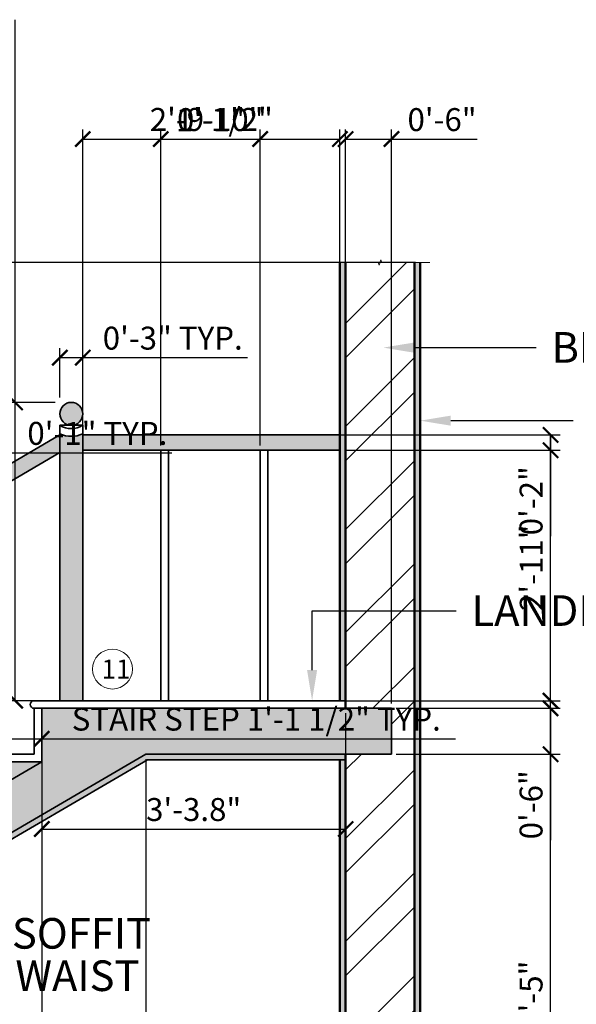
# Model space of a CAD drawing. Units: inches. Extents: x 2205 to 2524, y 4609 to 4803.
# Tile 4 of 5: x 2377 to 2450, y 4674 to 4803. Entities that reach past the tile are written whole.
import ezdxf
from ezdxf import colors
from ezdxf.entities.mleader import LeaderData, LeaderLine
from ezdxf.math import Vec2, Vec3

# ---------------------------------------------------------------- set-up
doc = ezdxf.new("R2010")
doc.units = ezdxf.units.IN
for name, color, linetype, lineweight in [('A-ANNO-DIMS', 2, 'Continuous', 18), ('A-ANNO-SYMB', 3, 'Continuous', 18), ('A-ANNO-TEXT', 7, 'Continuous', 18), ('A-FLOR-STRS', 7, 'Continuous', 35), ('A-SECT-PATT', 252, 'Continuous', 13), ('A-WALL', 1, 'Continuous', 50), ('A-WALL-PATT', 8, 'Continuous', 13), ('S-BEAM', 3, 'Continuous', 35)]:
    doc.layers.add(name, color=color, linetype=linetype, lineweight=lineweight)
doc.styles.get("Standard").update_dxf_attribs({"font": 'arial.ttf'})
doc.dimstyles.new('ISO-25', dxfattribs={"dimtxt": 3, "dimasz": 2, "dimexe": 1.25, "dimexo": 0.625, "dimtad": 1, "dimdec": 1, "dimlunit": 3, "dimtxsty": 'Standard', "dimblk": 'ARCHTICK', "dimcen": 2.5, "dimclrd": 5, "dimclre": 2, "dimclrt": 6, "dimadec": 0, "dimazin": 0, "dimtfac": 1, "dimtdec": 1, "dimtmove": 0, "dimatfit": 3, "dimfxl": 1, "dimarcsym": 0})

# ---------------------------------------------------------------- blocks, each defined once
blk = doc.blocks.new('_ArchTick')
at = {"color": 0, "linetype": 'ByBlock', "const_width": 0.15}
blk.add_lwpolyline([(-0.5, -0.5), (0.5, 0.5)], dxfattribs=at)
blk = doc.blocks.new('*D4')
at = {"layer": 'A-ANNO-DIMS', "color": 0, "lineweight": -2, "transparency": 16777216}
for p, q in [((2379.7, 4712.35), (2379.7, 4695.95)), ((2419.45, 4712.35), (2419.45, 4695.95)), ((2379.7, 4697.2), (2419.45, 4697.2))]:
    blk.add_line(p, q, dxfattribs=at)
at = {"layer": 'DEFPOINTS', "color": 0, "transparency": 16777216}
for p in [(2379.7, 4712.98), (2419.45, 4712.98), (2419.45, 4697.2)]:
    blk.add_point(p, dxfattribs=at)
at = {"layer": 'A-ANNO-DIMS', "color": 0, "lineweight": -2, "transparency": 16777216, "xscale": 2, "yscale": 2, "zscale": 2, "rotation": 180}
blk.add_blockref('_ArchTick', (2379.7, 4697.2), dxfattribs=at)
at = {"layer": 'A-ANNO-DIMS', "color": 0, "lineweight": -2, "transparency": 16777216, "xscale": 2, "yscale": 2, "zscale": 2}
blk.add_blockref('_ArchTick', (2419.45, 4697.2), dxfattribs=at)
at = {"layer": 'A-ANNO-DIMS', "color": 0, "transparency": 16777216, "insert": (2399.57, 4699.36), "char_height": 3, "attachment_point": 5}
blk.add_mtext('3\'-3.8"', dxfattribs=at)
blk = doc.blocks.new('STAIR-STEP')
for p, q in [((2282.7, 4650.98), (2270.7, 4650.98)), ((2283.7, 4649.98), (2270.7, 4649.98)), ((2270.7, 4649.98), (2270.7, 4642.98)), ((2271.7, 4649.98), (2271.7, 4642.98))]:
    blk.add_line(p, q)
blk.add_arc((2270.7, 4650.48), 0.5, 90, 270)
blk = doc.blocks.new('NEWEL-POST')
for p, q in [((2261.7, 4679.98), (2261.7, 4643.98)), ((2261.71, 4679.98), (2261.7, 4679.98)), ((2261.71, 4679.98), (2264.69, 4679.98)), ((2264.7, 4679.98), (2264.69, 4679.98)), ((2264.7, 4679.98), (2264.7, 4643.98))]:
    blk.add_line(p, q)
blk.add_circle((2263.2, 4681.48), 1.5)
for radius, start, end in [(2.78, 237.6128, 302.3872), (3.78, 246.6124, 293.3876)]:
    blk.add_arc((2263.2, 4682.33), radius, start, end)
blk = doc.blocks.new('*D9')
at = {"layer": 'A-ANNO-DIMS', "color": 2, "lineweight": -2, "transparency": 16777216}
for p, q in [((2366.2, 4707.6), (2366.2, 4710.25)), ((2379.7, 4707.6), (2379.7, 4710.25))]:
    blk.add_line(p, q, dxfattribs=at)
at = {"layer": 'A-ANNO-DIMS', "color": 5, "lineweight": -2, "transparency": 16777216}
for p, q in [((2366.2, 4709), (2379.7, 4709)), ((2379.7, 4709), (2433.83, 4709))]:
    blk.add_line(p, q, dxfattribs=at)
at = {"layer": 'DEFPOINTS', "color": 0, "transparency": 16777216}
for p in [(2379.7, 4709), (2366.2, 4706.98), (2379.7, 4706.98)]:
    blk.add_point(p, dxfattribs=at)
at = {"layer": 'A-ANNO-DIMS', "color": 5, "lineweight": -2, "transparency": 16777216, "xscale": 2, "yscale": 2, "zscale": 2, "rotation": 180}
blk.add_blockref('_ArchTick', (2366.2, 4709), dxfattribs=at)
at = {"layer": 'A-ANNO-DIMS', "color": 5, "lineweight": -2, "transparency": 16777216, "xscale": 2, "yscale": 2, "zscale": 2}
blk.add_blockref('_ArchTick', (2379.7, 4709), dxfattribs=at)
at = {"layer": 'A-ANNO-DIMS', "color": 6, "transparency": 16777216, "insert": (2407.76, 4711.18), "char_height": 3, "attachment_point": 5}
blk.add_mtext('STAIR STEP 1\'-1 1/2" TYP.', dxfattribs=at)
blk = doc.blocks.new('*D12')
at = {"layer": 'A-ANNO-DIMS', "color": 2, "lineweight": -2, "transparency": 16777216}
for p, q in [((2372.2, 4741.87), (2372.2, 4747.64)), ((2373.2, 4741.87), (2373.2, 4747.64))]:
    blk.add_line(p, q, dxfattribs=at)
at = {"layer": 'A-ANNO-DIMS', "color": 5, "lineweight": -2, "transparency": 16777216}
for p, q in [((2372.2, 4746.39), (2370.2, 4746.39)), ((2372.2, 4746.39), (2373.2, 4746.39)), ((2373.2, 4746.39), (2396.73, 4746.39))]:
    blk.add_line(p, q, dxfattribs=at)
at = {"layer": 'DEFPOINTS', "color": 0, "transparency": 16777216}
for p in [(2373.2, 4746.39), (2372.2, 4741.25), (2373.2, 4741.25)]:
    blk.add_point(p, dxfattribs=at)
at = {"layer": 'A-ANNO-DIMS', "color": 5, "lineweight": -2, "transparency": 16777216, "xscale": 2, "yscale": 2, "zscale": 2}
blk.add_blockref('_ArchTick', (2372.2, 4746.39), dxfattribs=at)
at = {"layer": 'A-ANNO-DIMS', "color": 5, "lineweight": -2, "transparency": 16777216, "xscale": 2, "yscale": 2, "zscale": 2, "rotation": 180}
blk.add_blockref('_ArchTick', (2373.2, 4746.39), dxfattribs=at)
at = {"layer": 'A-ANNO-DIMS', "color": 6, "transparency": 16777216, "insert": (2386.97, 4748.54), "char_height": 3, "attachment_point": 5}
blk.add_mtext('0\'-1" TYP.', dxfattribs=at)
blk = doc.blocks.new('*D13')
at = {"layer": 'A-ANNO-DIMS', "color": 5, "lineweight": -2, "transparency": 16777216}
for p, q in [((2376.21, 4752.98), (2376.21, 4803.01)), ((2376.21, 4713.98), (2376.21, 4752.98))]:
    blk.add_line(p, q, dxfattribs=at)
at = {"layer": 'A-ANNO-DIMS', "color": 2, "lineweight": -2, "transparency": 16777216}
for p, q in [((2381.44, 4752.98), (2374.96, 4752.98)), ((2381.44, 4713.98), (2374.96, 4713.98))]:
    blk.add_line(p, q, dxfattribs=at)
at = {"layer": 'DEFPOINTS', "color": 0, "transparency": 16777216}
for p in [(2376.21, 4752.98), (2382.06, 4752.98), (2382.06, 4713.98)]:
    blk.add_point(p, dxfattribs=at)
at = {"layer": 'A-ANNO-DIMS', "color": 5, "lineweight": -2, "transparency": 16777216, "xscale": 2, "yscale": 2, "zscale": 2}
for p, rotation in [((2376.21, 4752.98), 90), ((2376.21, 4713.98), 270)]:
    blk.add_blockref('_ArchTick', p, dxfattribs=dict(at, rotation=rotation))
at = {"layer": 'A-ANNO-DIMS', "color": 6, "transparency": 16777216, "insert": (2374.03, 4779), "char_height": 3, "attachment_point": 5, "rotation": 90}
blk.add_mtext('NEWEL POST 3\'-3" TYP.', dxfattribs=at)
blk = doc.blocks.new('*D14')
at = {"layer": 'A-ANNO-DIMS', "color": 2, "lineweight": -2, "transparency": 16777216}
for p, q in [((2382.06, 4753.6), (2382.06, 4760.08)), ((2385.06, 4753.6), (2385.06, 4760.08))]:
    blk.add_line(p, q, dxfattribs=at)
at = {"layer": 'A-ANNO-DIMS', "color": 5, "lineweight": -2, "transparency": 16777216}
for p, q in [((2382.06, 4758.83), (2385.06, 4758.83)), ((2385.06, 4758.83), (2406.6, 4758.83))]:
    blk.add_line(p, q, dxfattribs=at)
at = {"layer": 'DEFPOINTS', "color": 0, "transparency": 16777216}
for p in [(2385.06, 4758.83), (2382.06, 4752.98), (2385.06, 4752.98)]:
    blk.add_point(p, dxfattribs=at)
at = {"layer": 'A-ANNO-DIMS', "color": 5, "lineweight": -2, "transparency": 16777216, "xscale": 2, "yscale": 2, "zscale": 2, "rotation": 180}
blk.add_blockref('_ArchTick', (2382.06, 4758.83), dxfattribs=at)
at = {"layer": 'A-ANNO-DIMS', "color": 5, "lineweight": -2, "transparency": 16777216, "xscale": 2, "yscale": 2, "zscale": 2}
blk.add_blockref('_ArchTick', (2385.06, 4758.83), dxfattribs=at)
at = {"layer": 'A-ANNO-DIMS', "color": 6, "transparency": 16777216, "insert": (2396.83, 4760.99), "char_height": 3, "attachment_point": 5}
blk.add_mtext('0\'-3" TYP.', dxfattribs=at)
blk = doc.blocks.new('*D16')
at = {"layer": 'A-ANNO-DIMS', "color": 2, "lineweight": -2, "transparency": 16777216}
for p, q in [((2428.57, 4771.26), (2222.09, 4771.26)), ((2428.57, 4636.98), (2222.09, 4636.98))]:
    blk.add_line(p, q, dxfattribs=at)
at = {"layer": 'A-ANNO-DIMS', "color": 5, "lineweight": -2, "transparency": 16777216}
blk.add_line((2223.34, 4636.98), (2223.34, 4771.26), dxfattribs=at)
at = {"layer": 'DEFPOINTS', "color": 0, "transparency": 16777216}
for p in [(2223.34, 4771.26), (2429.2, 4771.26), (2429.2, 4636.98)]:
    blk.add_point(p, dxfattribs=at)
at = {"layer": 'A-ANNO-DIMS', "color": 5, "lineweight": -2, "transparency": 16777216, "xscale": 2, "yscale": 2, "zscale": 2}
for p, rotation in [((2223.34, 4771.26), 90), ((2223.34, 4636.98), 270)]:
    blk.add_blockref('_ArchTick', p, dxfattribs=dict(at, rotation=rotation))
at = {"layer": 'A-ANNO-DIMS', "color": 6, "transparency": 16777216, "insert": (2221.17, 4704.12), "char_height": 3, "attachment_point": 5, "rotation": 90}
blk.add_mtext('11\'-2 1/2"', dxfattribs=at)
blk = doc.blocks.new('*D17')
at = {"layer": 'A-ANNO-DIMS', "color": 2, "lineweight": -2, "transparency": 16777216}
for p, q in [((2420.07, 4713.98), (2447.5, 4713.98)), ((2420.07, 4636.98), (2447.5, 4636.98))]:
    blk.add_line(p, q, dxfattribs=at)
at = {"layer": 'A-ANNO-DIMS', "color": 5, "lineweight": -2, "transparency": 16777216}
blk.add_line((2446.25, 4636.98), (2446.25, 4713.98), dxfattribs=at)
at = {"layer": 'DEFPOINTS', "color": 0, "transparency": 16777216}
for p in [(2419.45, 4713.98), (2446.25, 4713.98), (2419.45, 4636.98)]:
    blk.add_point(p, dxfattribs=at)
at = {"layer": 'A-ANNO-DIMS', "color": 5, "lineweight": -2, "transparency": 16777216, "xscale": 2, "yscale": 2, "zscale": 2}
for p, rotation in [((2446.25, 4713.98), 90), ((2446.25, 4636.98), 270)]:
    blk.add_blockref('_ArchTick', p, dxfattribs=dict(at, rotation=rotation))
at = {"layer": 'A-ANNO-DIMS', "color": 6, "transparency": 16777216, "insert": (2444.09, 4675.48), "char_height": 3, "attachment_point": 5, "rotation": 90}
blk.add_mtext('6\'-5"', dxfattribs=at)
blk = doc.blocks.new('*D19')
at = {"layer": 'A-ANNO-DIMS', "color": 2, "lineweight": -2, "transparency": 16777216}
for p, q in [((2426.07, 4712.98), (2447.5, 4712.98)), ((2426.07, 4706.98), (2447.5, 4706.98))]:
    blk.add_line(p, q, dxfattribs=at)
at = {"layer": 'A-ANNO-DIMS', "color": 5, "lineweight": -2, "transparency": 16777216}
for p, q in [((2446.25, 4712.98), (2446.25, 4706.98)), ((2446.25, 4706.98), (2446.25, 4695.75))]:
    blk.add_line(p, q, dxfattribs=at)
at = {"layer": 'DEFPOINTS', "color": 0, "transparency": 16777216}
for p in [(2425.45, 4712.98), (2425.45, 4706.98), (2446.25, 4706.98)]:
    blk.add_point(p, dxfattribs=at)
at = {"layer": 'A-ANNO-DIMS', "color": 5, "lineweight": -2, "transparency": 16777216, "xscale": 2, "yscale": 2, "zscale": 2}
for p, rotation in [((2446.25, 4712.98), 90), ((2446.25, 4706.98), 270)]:
    blk.add_blockref('_ArchTick', p, dxfattribs=dict(at, rotation=rotation))
at = {"layer": 'A-ANNO-DIMS', "color": 6, "transparency": 16777216, "insert": (2444.09, 4700.37), "char_height": 3, "attachment_point": 5, "rotation": 90}
blk.add_mtext('0\'-6"', dxfattribs=at)
blk = doc.blocks.new('*D20')
at = {"layer": 'A-ANNO-DIMS', "color": 2, "lineweight": -2, "transparency": 16777216}
for p, q in [((2419.45, 4713.6), (2419.45, 4788.66)), ((2425.45, 4713.6), (2425.45, 4788.66))]:
    blk.add_line(p, q, dxfattribs=at)
at = {"layer": 'A-ANNO-DIMS', "color": 5, "lineweight": -2, "transparency": 16777216}
for p, q in [((2419.45, 4787.41), (2425.45, 4787.41)), ((2425.45, 4787.41), (2436.67, 4787.41))]:
    blk.add_line(p, q, dxfattribs=at)
at = {"layer": 'DEFPOINTS', "color": 0, "transparency": 16777216}
for p in [(2425.45, 4787.41), (2419.45, 4712.98), (2425.45, 4712.98)]:
    blk.add_point(p, dxfattribs=at)
at = {"layer": 'A-ANNO-DIMS', "color": 5, "lineweight": -2, "transparency": 16777216, "xscale": 2, "yscale": 2, "zscale": 2, "rotation": 180}
blk.add_blockref('_ArchTick', (2419.45, 4787.41), dxfattribs=at)
at = {"layer": 'A-ANNO-DIMS', "color": 5, "lineweight": -2, "transparency": 16777216, "xscale": 2, "yscale": 2, "zscale": 2}
blk.add_blockref('_ArchTick', (2425.45, 4787.41), dxfattribs=at)
at = {"layer": 'A-ANNO-DIMS', "color": 6, "transparency": 16777216, "insert": (2432.06, 4789.56), "char_height": 3, "attachment_point": 5}
blk.add_mtext('0\'-6"', dxfattribs=at)
blk = doc.blocks.new('*D21')
at = {"layer": 'A-ANNO-DIMS', "color": 2, "lineweight": -2, "transparency": 16777216}
for p, q in [((2379.7, 4705.35), (2379.7, 4619.93)), ((2393.32, 4706.35), (2393.32, 4619.93))]:
    blk.add_line(p, q, dxfattribs=at)
at = {"layer": 'A-ANNO-DIMS', "color": 5, "lineweight": -2, "transparency": 16777216}
for p, q in [((2379.7, 4621.18), (2393.32, 4621.18)), ((2393.32, 4621.18), (2411.25, 4621.18))]:
    blk.add_line(p, q, dxfattribs=at)
at = {"layer": 'DEFPOINTS', "color": 0, "transparency": 16777216}
for p in [(2393.32, 4706.98), (2379.7, 4705.98), (2393.32, 4621.18)]:
    blk.add_point(p, dxfattribs=at)
at = {"layer": 'A-ANNO-DIMS', "color": 5, "lineweight": -2, "transparency": 16777216, "xscale": 2, "yscale": 2, "zscale": 2, "rotation": 180}
blk.add_blockref('_ArchTick', (2379.7, 4621.18), dxfattribs=at)
at = {"layer": 'A-ANNO-DIMS', "color": 5, "lineweight": -2, "transparency": 16777216, "xscale": 2, "yscale": 2, "zscale": 2}
blk.add_blockref('_ArchTick', (2393.32, 4621.18), dxfattribs=at)
at = {"layer": 'A-ANNO-DIMS', "color": 6, "transparency": 16777216, "insert": (2403.29, 4623.36), "char_height": 3, "attachment_point": 5}
blk.add_mtext('1\'-1 1/2"', dxfattribs=at)
blk = doc.blocks.new('*D22')
at = {"layer": 'A-ANNO-DIMS', "color": 2, "lineweight": -2, "transparency": 16777216}
for p, q in [((2385.69, 4748.73), (2447.5, 4748.73)), ((2385.69, 4713.98), (2447.5, 4713.98))]:
    blk.add_line(p, q, dxfattribs=at)
at = {"layer": 'A-ANNO-DIMS', "color": 5, "lineweight": -2, "transparency": 16777216}
blk.add_line((2446.25, 4713.98), (2446.25, 4748.73), dxfattribs=at)
at = {"layer": 'DEFPOINTS', "color": 0, "transparency": 16777216}
for p in [(2385.06, 4748.73), (2446.25, 4748.73), (2385.06, 4713.98)]:
    blk.add_point(p, dxfattribs=at)
at = {"layer": 'A-ANNO-DIMS', "color": 5, "lineweight": -2, "transparency": 16777216, "xscale": 2, "yscale": 2, "zscale": 2}
for p, rotation in [((2446.25, 4748.73), 90), ((2446.25, 4713.98), 270)]:
    blk.add_blockref('_ArchTick', p, dxfattribs=dict(at, rotation=rotation))
at = {"layer": 'A-ANNO-DIMS', "color": 6, "transparency": 16777216, "insert": (2444.12, 4731.36), "char_height": 3, "attachment_point": 5, "rotation": 90}
blk.add_mtext('2\'-11"', dxfattribs=at)
blk = doc.blocks.new('*D23')
at = {"layer": 'A-ANNO-DIMS', "color": 2, "lineweight": -2, "transparency": 16777216}
for p, q in [((2419.32, 4748.73), (2447.5, 4748.73)), ((2419.32, 4746.73), (2447.5, 4746.73))]:
    blk.add_line(p, q, dxfattribs=at)
at = {"layer": 'A-ANNO-DIMS', "color": 5, "lineweight": -2, "transparency": 16777216}
for p, q in [((2446.25, 4748.73), (2446.25, 4746.73)), ((2446.25, 4746.73), (2446.25, 4735.51))]:
    blk.add_line(p, q, dxfattribs=at)
at = {"layer": 'DEFPOINTS', "color": 0, "transparency": 16777216}
for p in [(2418.7, 4748.73), (2418.7, 4746.73), (2446.25, 4746.73)]:
    blk.add_point(p, dxfattribs=at)
at = {"layer": 'A-ANNO-DIMS', "color": 5, "lineweight": -2, "transparency": 16777216, "xscale": 2, "yscale": 2, "zscale": 2}
for p, rotation in [((2446.25, 4748.73), 90), ((2446.25, 4746.73), 270)]:
    blk.add_blockref('_ArchTick', p, dxfattribs=dict(at, rotation=rotation))
at = {"layer": 'A-ANNO-DIMS', "color": 6, "transparency": 16777216, "insert": (2444.09, 4740.12), "char_height": 3, "attachment_point": 5, "rotation": 90}
blk.add_mtext('0\'-2"', dxfattribs=at)
blk = doc.blocks.new('*D25')
at = {"layer": 'A-ANNO-DIMS', "color": 2, "lineweight": -2, "transparency": 16777216}
for p, q in [((2385.06, 4750.6), (2385.06, 4788.66)), ((2418.7, 4749.36), (2418.7, 4788.66))]:
    blk.add_line(p, q, dxfattribs=at)
at = {"layer": 'A-ANNO-DIMS', "color": 5, "lineweight": -2, "transparency": 16777216}
blk.add_line((2385.06, 4787.41), (2418.7, 4787.41), dxfattribs=at)
at = {"layer": 'DEFPOINTS', "color": 0, "transparency": 16777216}
for p in [(2418.7, 4787.41), (2385.06, 4749.98), (2418.7, 4748.73)]:
    blk.add_point(p, dxfattribs=at)
at = {"layer": 'A-ANNO-DIMS', "color": 5, "lineweight": -2, "transparency": 16777216, "xscale": 2, "yscale": 2, "zscale": 2, "rotation": 180}
blk.add_blockref('_ArchTick', (2385.06, 4787.41), dxfattribs=at)
at = {"layer": 'A-ANNO-DIMS', "color": 5, "lineweight": -2, "transparency": 16777216, "xscale": 2, "yscale": 2, "zscale": 2}
blk.add_blockref('_ArchTick', (2418.7, 4787.41), dxfattribs=at)
at = {"layer": 'A-ANNO-DIMS', "color": 6, "transparency": 16777216, "insert": (2401.88, 4789.58), "char_height": 3, "attachment_point": 5}
blk.add_mtext('2\'-9 1/2"', dxfattribs=at)
blk = doc.blocks.new('*D35')
at = {"layer": 'A-ANNO-DIMS', "color": 2, "lineweight": -2, "transparency": 16777216}
for p, q in [((2385.06, 4747.36), (2385.06, 4788.66)), ((2395.26, 4747.36), (2395.26, 4788.66))]:
    blk.add_line(p, q, dxfattribs=at)
at = {"layer": 'A-ANNO-DIMS', "color": 5, "lineweight": -2, "transparency": 16777216}
for p, q in [((2385.06, 4787.41), (2395.26, 4787.41)), ((2395.26, 4787.41), (2408.82, 4787.41))]:
    blk.add_line(p, q, dxfattribs=at)
at = {"layer": 'DEFPOINTS', "color": 0, "transparency": 16777216}
for p in [(2395.26, 4787.41), (2385.06, 4746.73), (2395.26, 4746.73)]:
    blk.add_point(p, dxfattribs=at)
at = {"layer": 'A-ANNO-DIMS', "color": 5, "lineweight": -2, "transparency": 16777216, "xscale": 2, "yscale": 2, "zscale": 2, "rotation": 180}
blk.add_blockref('_ArchTick', (2385.06, 4787.41), dxfattribs=at)
at = {"layer": 'A-ANNO-DIMS', "color": 5, "lineweight": -2, "transparency": 16777216, "xscale": 2, "yscale": 2, "zscale": 2}
blk.add_blockref('_ArchTick', (2395.26, 4787.41), dxfattribs=at)
at = {"layer": 'A-ANNO-DIMS', "color": 6, "transparency": 16777216, "insert": (2403.04, 4789.56), "char_height": 3, "attachment_point": 5}
blk.add_mtext('0\'-10"', dxfattribs=at)
blk = doc.blocks.new('*D36')
at = {"layer": 'A-ANNO-DIMS', "color": 2, "lineweight": -2, "transparency": 16777216}
for p, q in [((2395.26, 4747.36), (2395.26, 4788.66)), ((2408.26, 4747.36), (2408.26, 4788.66))]:
    blk.add_line(p, q, dxfattribs=at)
at = {"layer": 'A-ANNO-DIMS', "color": 5, "lineweight": -2, "transparency": 16777216}
blk.add_line((2395.26, 4787.41), (2408.26, 4787.41), dxfattribs=at)
at = {"layer": 'DEFPOINTS', "color": 0, "transparency": 16777216}
for p in [(2408.26, 4787.41), (2395.26, 4746.73), (2408.26, 4746.73)]:
    blk.add_point(p, dxfattribs=at)
at = {"layer": 'A-ANNO-DIMS', "color": 5, "lineweight": -2, "transparency": 16777216, "xscale": 2, "yscale": 2, "zscale": 2, "rotation": 180}
blk.add_blockref('_ArchTick', (2395.26, 4787.41), dxfattribs=at)
at = {"layer": 'A-ANNO-DIMS', "color": 5, "lineweight": -2, "transparency": 16777216, "xscale": 2, "yscale": 2, "zscale": 2}
blk.add_blockref('_ArchTick', (2408.26, 4787.41), dxfattribs=at)
at = {"layer": 'A-ANNO-DIMS', "color": 6, "transparency": 16777216, "insert": (2401.76, 4789.54), "char_height": 3, "attachment_point": 5}
blk.add_mtext('1\'-1"', dxfattribs=at)

msp = doc.modelspace()

# ---------------------------------------------------------------- hatches: boundary and pattern name
at = {"layer": 'A-SECT-PATT'}
h = msp.add_hatch(dxfattribs=at)
h.set_pattern_fill('AR-CONC', color=256, scale=0.04)
h.paths.add_polyline_path([(2393.32, 4706.98), (2419.45, 4706.98), (2425.45, 4706.98), (2425.45, 4712.98), (2419.45, 4712.98), (2379.7, 4712.98), (2379.7, 4705.98), (2271.7, 4642.98), (2259.7, 4636.98), (2273.32, 4636.98)])
h.paths.add_polyline_path([(2343.7, 4684.98), (2331.7, 4684.98), (2331.7, 4677.98)], flags=16)
h.paths.add_polyline_path([(2331.7, 4677.98), (2319.7, 4677.98), (2319.7, 4670.98)], flags=16)
h.paths.add_polyline_path([(2319.7, 4670.98), (2307.7, 4670.98), (2307.7, 4663.98)], flags=16)
h.paths.add_polyline_path([(2307.7, 4663.98), (2295.7, 4663.98), (2295.7, 4656.98)], flags=16)
h.paths.add_polyline_path([(2295.7, 4656.98), (2283.7, 4656.98), (2283.7, 4649.98)], flags=16)
h.paths.add_polyline_path([(2283.7, 4649.98), (2271.7, 4649.98), (2271.7, 4642.98)], flags=17)
h.paths.add_polyline_path([(2271.7, 4642.98), (2259.7, 4642.98), (2259.7, 4636.98)], flags=17)
h.paths.add_polyline_path([(2379.7, 4705.98), (2367.7, 4705.98), (2367.7, 4698.98)], flags=16)
h.paths.add_polyline_path([(2367.7, 4698.98), (2355.7, 4698.98), (2355.7, 4691.98)], flags=16)
h.paths.add_polyline_path([(2419.45, 4706.98), (2393.32, 4706.98), (2273.32, 4636.98), (2274.81, 4636.98), (2393.52, 4706.23), (2419.45, 4706.23)], flags=17)
h.paths.add_polyline_path([(2419.45, 4706.23), (2418.7, 4706.23), (2418.7, 4636.98), (2419.45, 4636.98)], flags=16)
h.paths.add_polyline_path([(2429.2, 4771.26), (2428.45, 4771.26), (2428.45, 4636.98), (2429.2, 4636.98)])
h.paths.add_polyline_path([(2419.45, 4771.26), (2418.7, 4771.26), (2418.7, 4713.98), (2419.45, 4713.98)])
h = msp.add_hatch(color=256, dxfattribs=at)
h.dxf.hatch_style = 1
h.paths.add_polyline_path([(2264.7, 4678.86, -0.206977), (2261.7, 4678.86), (2261.7, 4643.98), (2264.7, 4643.98)])
h.paths.add_polyline_path([(2261.7, 4681.48, 1), (2264.7, 4681.48, 1)])
h.paths.add_polyline_path([(2382.06, 4746.42), (2382.06, 4748.73), (2264.2, 4679.98), (2264.69, 4679.98), (2264.7, 4679.98), (2264.7, 4677.96)])
h.paths.add_polyline_path([(2418.7, 4748.73), (2385.06, 4748.73), (2385.06, 4746.73), (2418.7, 4746.73)])
h.paths.add_polyline_path([(2385.06, 4748.86, -0.206977), (2382.06, 4748.86), (2382.06, 4713.98), (2385.06, 4713.98)])
h.paths.add_polyline_path([(2382.06, 4751.48, 1), (2385.06, 4751.48, 1)])
at = {"layer": 'A-WALL-PATT'}
h = msp.add_hatch(dxfattribs=at)
h.set_pattern_fill('ANSI32', color=256)
h.paths.add_polyline_path([(2428.45, 4771.26), (2419.45, 4771.26), (2419.45, 4712.98), (2425.45, 4712.98), (2425.45, 4706.98), (2419.45, 4706.98), (2419.45, 4636.98), (2428.45, 4636.98)])

# ---------------------------------------------------------------- linework, layer by layer
at = {"layer": 'A-ANNO-SYMB'}
msp.add_lwpolyline([(2417.45, 4771.26), (2423.7, 4771.26), (2423.82, 4770.92), (2424.07, 4771.61), (2424.2, 4771.26), (2430.45, 4771.26)], dxfattribs=at)
msp.add_circle((2388.95, 4718.11), 2.61, dxfattribs=at)
at = {"layer": 'A-FLOR-STRS'}
for p, q in [((2384.76, 4749.98), (2382.06, 4749.98)), ((2264.2, 4679.98), (2382.06, 4748.73)), ((2385.06, 4748.73), (2418.7, 4748.73)), ((2264.7, 4677.96), (2382.06, 4746.42)), ((2385.06, 4746.73), (2418.7, 4746.73)), ((2395.26, 4746.73), (2395.26, 4713.98)), ((2396.26, 4746.73), (2396.26, 4713.98)), ((2408.26, 4746.73), (2408.26, 4713.98)), ((2409.26, 4746.73), (2409.26, 4713.98)), ((2378.7, 4712.98), (2378.7, 4706.98)), ((2379.7, 4712.98), (2379.7, 4705.98)), ((2273.32, 4636.98), (2393.32, 4706.98)), ((2271.7, 4642.98), (2379.7, 4705.98)), ((2274.81, 4636.98), (2393.52, 4706.23))]:
    msp.add_line(p, q, dxfattribs=at)
msp.add_arc((2378.7, 4713.48), 0.5, 90, 270, dxfattribs=at)
at = {"layer": 'A-WALL'}
for p, q in [((2418.7, 4771.26), (2418.7, 4713.98)), ((2419.45, 4771.26), (2419.45, 4712.98)), ((2428.45, 4771.26), (2428.45, 4636.98)), ((2429.2, 4771.26), (2429.2, 4636.98)), ((2419.45, 4706.98), (2419.45, 4636.98)), ((2418.7, 4706.23), (2418.7, 4636.98))]:
    msp.add_line(p, q, dxfattribs=at)
at = {"layer": 'S-BEAM'}
for p, q in [((2378.7, 4713.98), (2419.45, 4713.98)), ((2378.7, 4712.98), (2379.7, 4712.98)), ((2379.7, 4712.98), (2419.45, 4712.98)), ((2419.45, 4712.98), (2425.45, 4712.98)), ((2425.45, 4712.98), (2425.45, 4706.98)), ((2393.32, 4706.98), (2419.45, 4706.98)), ((2425.45, 4706.98), (2419.45, 4706.98)), ((2393.52, 4706.23), (2419.45, 4706.23))]:
    msp.add_line(p, q, dxfattribs=at)

# ---------------------------------------------------------------- block references
at = {"layer": 'A-FLOR-STRS'}
for name, p in [('NEWEL-POST', (120.36, 70)), ('STAIR-STEP', (96, 56))]:
    msp.add_blockref(name, p, dxfattribs=at)

# ---------------------------------------------------------------- texts
at = {"layer": 'A-ANNO-TEXT', "insert": (2387.52, 4719.36), "char_height": 2.5, "attachment_point": 1}
msp.add_mtext_dynamic_manual_height_columns('11', width=3.6522, gutter_width=12.5, heights=[0], dxfattribs=at)

# ---------------------------------------------------------------- dimensions: what is measured, and where the dimension line sits
at = {"layer": 'A-ANNO-DIMS'}
dim = msp.add_linear_dim(base=(2376.21, 4752.98), p1=(2382.06, 4713.98), p2=(2382.06, 4752.98), angle=90, text='NEWEL POST <> TYP.', dimstyle='ISO-25', override={"dimdec": 1, "dimrnd": 0, "dimzin": 1, "dimlunit": 4, "dimfrac": 2}, dxfattribs=at)
dim.commit()
dim.dimension.update_dxf_attribs({"geometry": '*D13', "text_midpoint": (2374.03, 4779)})
for base, p1, p2, override, picture, middle in [((2418.7, 4787.41), (2385.06, 4749.98), (2418.7, 4748.73), {"dimdec": 1, "dimlfac": 1, "dimrnd": 0, "dimzin": 1, "dimdsep": 46, "dimlunit": 4, "dimfrac": 2}, '*D25', (2401.88, 4789.58)), ((2395.26, 4787.41), (2385.06, 4746.73), (2395.26, 4746.73), {"dimdec": 1, "dimlfac": 1, "dimrnd": 0, "dimzin": 1, "dimdsep": 46, "dimlunit": 4, "dimfrac": 2}, '*D35', (2403.04, 4789.56)), ((2408.26, 4787.41), (2395.26, 4746.73), (2408.26, 4746.73), {"dimdec": 1, "dimlfac": 1, "dimrnd": 0, "dimzin": 1, "dimdsep": 46, "dimlunit": 4, "dimfrac": 2}, '*D36', (2401.76, 4789.54)), ((2425.45, 4787.41), (2419.45, 4712.98), (2425.45, 4712.98), {"dimdec": 1, "dimlfac": 1, "dimrnd": 0, "dimzin": 1, "dimdsep": 46, "dimlunit": 4, "dimfrac": 2}, '*D20', (2432.06, 4789.56)), ((2419.44688598, 4697.20138406), (2379.69688598, 4712.97926808), (2419.44688598, 4712.97926808), {"dimclrd": 0, "dimclre": 0, "dimclrt": 0}, '*D4', (2399.57188598, 4699.35912621)), ((2393.32, 4621.18), (2379.7, 4705.98), (2393.32, 4706.98), {"dimdec": 1, "dimlfac": 1, "dimrnd": 0, "dimzin": 1, "dimdsep": 46, "dimlunit": 4, "dimfrac": 2}, '*D21', (2403.29, 4623.36))]:
    dim = msp.add_linear_dim(base=base, p1=p1, p2=p2, dimstyle='ISO-25', override=override, dxfattribs=at)
    dim.commit()
    dim.dimension.update_dxf_attribs({"geometry": picture, "text_midpoint": middle})
for base, p1, p2, picture, middle in [((2223.34, 4771.26), (2429.2, 4636.98), (2429.2, 4771.26), '*D16', (2221.17, 4704.12)), ((2446.2469, 4748.7336), (2385.0614, 4713.9793), (2385.0614, 4748.7336), '*D22', (2444.1157, 4731.3564)), ((2446.25, 4746.73), (2418.7, 4748.73), (2418.7, 4746.73), '*D23', (2444.09, 4740.12)), ((2446.25, 4713.98), (2419.45, 4636.98), (2419.45, 4713.98), '*D17', (2444.09, 4675.48)), ((2446.25, 4706.98), (2425.45, 4712.98), (2425.45, 4706.98), '*D19', (2444.09, 4700.37))]:
    dim = msp.add_linear_dim(base=base, p1=p1, p2=p2, angle=90, dimstyle='ISO-25', override={"dimdec": 1, "dimlfac": 1, "dimrnd": 0, "dimzin": 1, "dimdsep": 46, "dimlunit": 4, "dimfrac": 2}, dxfattribs=at)
    dim.commit()
    dim.dimension.update_dxf_attribs({"geometry": picture, "text_midpoint": middle})
for base, p1, p2, text, picture, middle in [((2385.06, 4758.83), (2382.06, 4752.98), (2385.06, 4752.98), '<> TYP.', '*D14', (2396.83, 4760.99)), ((2373.2, 4746.39), (2372.2, 4741.25), (2373.2, 4741.25), '<> TYP.', '*D12', (2386.97, 4748.54)), ((2379.7, 4709), (2366.2, 4706.98), (2379.7, 4706.98), 'STAIR STEP <> TYP.', '*D9', (2407.76, 4711.18))]:
    dim = msp.add_linear_dim(base=base, p1=p1, p2=p2, text=text, dimstyle='ISO-25', override={"dimdec": 1, "dimrnd": 0, "dimzin": 1, "dimlunit": 4, "dimfrac": 2}, dxfattribs=at)
    dim.commit()
    dim.dimension.update_dxf_attribs({"geometry": picture, "text_midpoint": middle})

# ---------------------------------------------------------------- leaders
at = {"layer": 'A-ANNO-SYMB'}
ml = msp.add_multileader_mtext('Standard', dxfattribs=at)
ml.set_content('BRICK WALL-9"', color=256)
ml.set_leader_properties()
ml.build(insert=Vec2(0, 0))
ctx = ml.context
ctx.base_point, ctx.plane_origin = Vec3(2444.38, 4760.14), Vec3(2424.36, 4760.14)
notes = []
notes.append((ctx, [(0, (1, 1, 0), (2436.38, 4760.14), (1, 0), 8, [(0, [(2424.36, 4760.14)], 0, [])])]))
ctx.mtext.insert, ctx.mtext.width, ctx.mtext.flow_direction = Vec3(2446.38, 4762.17), 53.5271, 5
ml = msp.add_multileader_mtext('Standard', dxfattribs=at)
ml.set_content('CEMENT PLASTER-.75"', color=256)
ml.set_leader_properties()
ml.build(insert=Vec2(0, 0))
ctx = ml.context
ctx.base_point, ctx.plane_origin = Vec3(2449.22, 4750.59), Vec3(2429.2, 4750.59)
notes.append((ctx, [(0, (1, 1, 0), (2441.22, 4750.59), (1, 0), 8, [(0, [(2429.2, 4750.59)], 0, [])])]))
ctx.mtext.insert, ctx.mtext.width, ctx.mtext.flow_direction = Vec3(2451.22, 4752.62), 72.3695, 5
ml = msp.add_multileader_mtext('Standard', dxfattribs=at)
ml.set_content('LANDING', color=256)
ml.set_leader_properties()
ml.build(insert=Vec2(0, 0))
ctx = ml.context
ctx.base_point, ctx.plane_origin = Vec3(2433.91, 4725.73), Vec3(2415.06, 4713.98)
notes.append((ctx, [(0, (1, 1, 0), (2415.06, 4725.73), (1, 0), 18.85, [(0, [(2415.06, 4713.98)], 0, [])])]))
ctx.mtext.insert, ctx.mtext.width, ctx.mtext.flow_direction = Vec3(2435.91, 4727.76), 24.3641, 5
ml = msp.add_multileader_mtext('Standard', dxfattribs=at)
ml.set_content('SOFFIT', color=256)
ml.set_leader_properties()
ml.build(insert=Vec2(0, 0))
ctx = ml.context
ctx.base_point, ctx.plane_origin = Vec3(2373.8, 4683.53), Vec3(2353.78, 4683.53)
notes.append((ctx, [(0, (1, 1, 0), (2365.8, 4683.53), (1, 0), 8, [(0, [(2353.78, 4683.53)], 0, [])])]))
ctx.mtext.insert, ctx.mtext.width, ctx.mtext.flow_direction = Vec3(2375.8, 4685.56), 53.5271, 5
ml = msp.add_multileader_mtext('Standard', dxfattribs=at)
ml.set_content('WAIST', color=256)
ml.set_leader_properties()
ml.build(insert=Vec2(0, 0))
ctx = ml.context
ctx.base_point, ctx.plane_origin = Vec3(2374.25, 4677.99), Vec3(2340.01, 4677.99)
notes.append((ctx, [(0, (1, 1, 0), (2352.03, 4677.99), (1, 0), 22.22, [(0, [(2340.01, 4677.99)], 0, [])])]))
ctx.mtext.insert, ctx.mtext.width, ctx.mtext.flow_direction = Vec3(2376.25, 4680.02), 53.5271, 5
for ctx, leaders in notes:
    for number, flags, end, landing, length, lines in leaders:
        leader = LeaderData()
        leader.index, (leader.has_last_leader_line, leader.has_dogleg_vector, leader.attachment_direction) = number, flags
        leader.last_leader_point, leader.dogleg_vector, leader.dogleg_length = Vec3(end), Vec3(landing), length
        for number, points, colour, breaks in lines:
            line = LeaderLine()
            line.index, line.vertices, line.color, line.breaks = number, Vec3.list(points), colors.encode_raw_color(colour), breaks
            leader.lines.append(line)
        ctx.leaders.append(leader)

doc.saveas('drawing.dxf')
